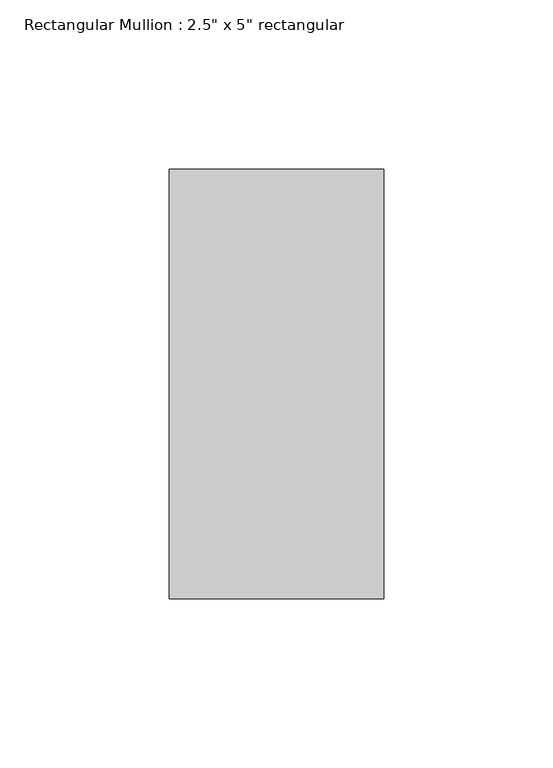
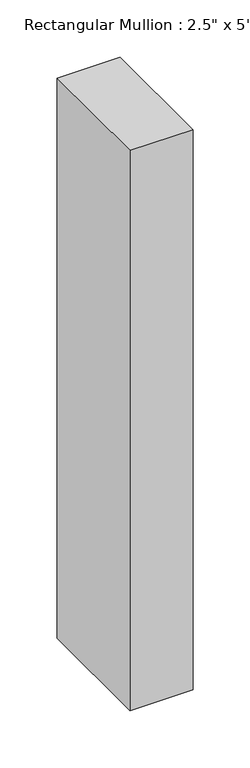
"""IFC4 building model written with IfcOpenShell, lengths in millimetres: member geometry."""

from ifc_helpers import new_model, si_unit, frame, origin, place, context, project, spatial, polyline, outline, extrude, source, transform, mapped, element, save


def member_86293703(model_context):
    return source(origin(), model_context, "Body", "SweptSolid", [
        extrude(outline(polyline([(31.75, 63.5), (31.75, -63.5), (-31.75, -63.5), (-31.75, 63.5), (31.75, 63.5)])), frame((0.0, 0.0, -596.9), z_axis=(0.0, 0.0, 1.0), x_axis=(1.0, 0.0, 0.0)), (0.0, 0.0, 1.0), 596.9),
    ])


if __name__ == "__main__":
    model = new_model("IFC4")
    model_context = context("Model", 3, world=origin())
    ifc_project = project(units=[si_unit("LENGTHUNIT", "METRE", prefix="MILLI")], contexts=[model_context])
    site = spatial("IfcSite", under=ifc_project)
    building = spatial("IfcBuilding", under=site)
    placement = place(None, origin())
    member_shape = member_86293703(model_context)
    element("IfcMember", 1, ObjectType="Rectangular Mullion : 2.5\" x 5\" rectangular", at=placement, inside=building, context=model_context, shape_type="MappedRepresentation", body=[
        mapped(member_shape, transform((0.0, 0.0, 0.0), x_axis=(1.0, 0.0, 0.0), y_axis=(0.0, 1.0, 0.0), z_axis=(0.0, 0.0, 1.0))),
    ])
    save(model, "model.ifc")

# Revit data of these elements
# Type "Rectangular Mullion : 2.5\" x 5\" rectangular"
#   built-in parameter 1007304 = 0.416667 (stored number, unit not read)
#   built-in parameter 1007301 = 0.104167 (stored number, unit not read)
#   built-in parameter 1007300 = 0.104167 (stored number, unit not read)
# Element 1 (IfcMember, "Rectangular Mullion : 2.5\" x 5\" rectangular")
#   Materials on its faces: "Aluminum"
# Materials
#   "Aluminum": class "Metal", colour RGB 247 247 247, transparency 0, Description = "Aluminum 6061", Cost = 0
